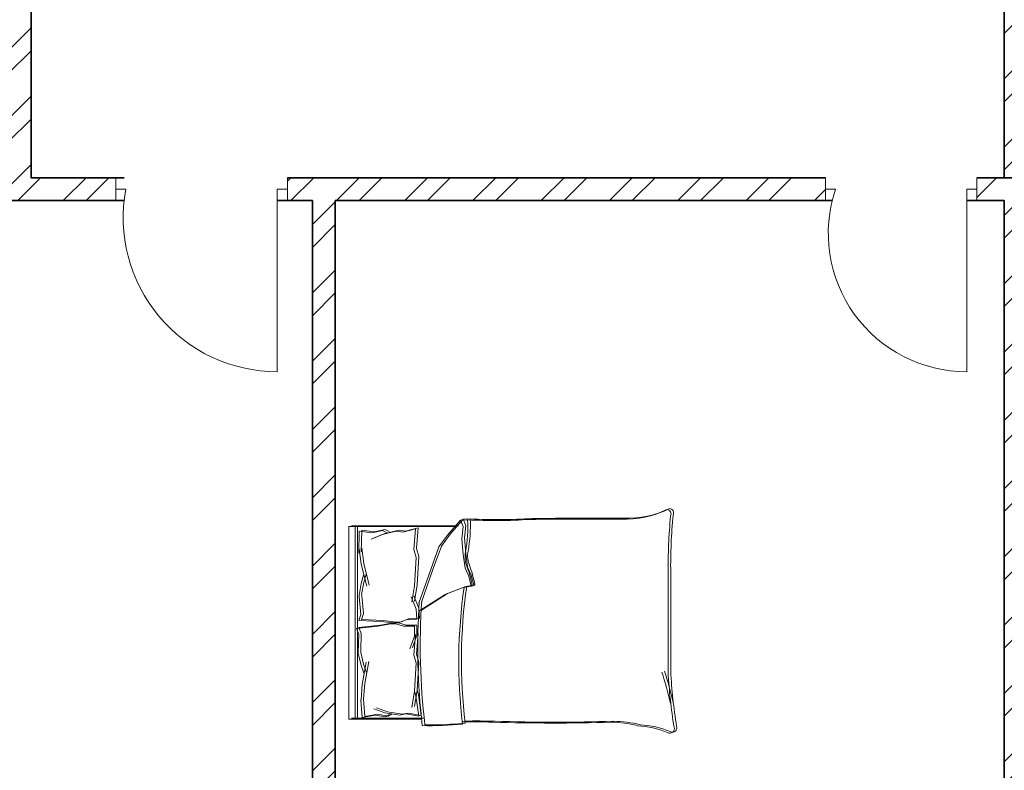
# Model space of a CAD drawing. Units: inches. Extents: x 1962 to 2771, y 1245 to 2660.
# Tile 3 of 114: x 2177 to 2371, y 1534 to 1683. Entities that reach past the tile are written whole.
import ezdxf

# ---------------------------------------------------------------- set-up
doc = ezdxf.new("R2010")
doc.units = ezdxf.units.IN
for name, color, linetype, lineweight in [('A-DOOR', 3, 'Continuous', 18), ('A-FURN', 8, 'Continuous', 13), ('A-WALL', 7, 'Continuous', 35), ('A-WALL-PATT', 252, 'Continuous', 13)]:
    doc.layers.add(name, color=color, linetype=linetype, lineweight=lineweight)

# ---------------------------------------------------------------- blocks, each defined once
blk = doc.blocks.new('BED-PLAN')
for p, q in [((0.51, 40.93), (21.66, 40.93)), ((0.51, 40.93), (21.66, 40.93)), ((1.73, 2.95), (1.73, 40.93)), ((1.73, 2.95), (1.73, 40.93)), ((22.05, 42.03), (19.47, 39.08)), ((22.05, 42.02), (19.47, 39.08)), ((22.56, 42.21), (19.98, 39.26)), ((22.56, 42.21), (19.98, 39.26)), ((23.44, 42.09), (22.05, 42.03, 3.08)), ((23.44, 42.09), (22.05, 42.02, 3.08)), ((22.55, 40.8), (22.05, 42.03)), ((22.55, 40.8), (22.05, 42.02)), ((22.3, 38.34), (22.55, 40.8)), ((22.3, 38.34), (22.55, 40.8)), ((23.95, 42.27), (22.56, 42.21, 3.08)), ((23.95, 42.27), (22.56, 42.21, 3.08)), ((23.06, 40.98), (22.56, 42.21)), ((23.06, 40.98), (22.56, 42.21)), ((22.81, 38.52), (23.06, 40.98)), ((22.81, 38.52), (23.06, 40.98)), ((0, 40.75), (21.15, 40.75)), ((0, 40.75), (21.15, 40.75)), ((0, 2.76), (0, 40.75)), ((1.22, 2.76), (1.22, 40.75)), ((1.22, 2.76), (1.22, 40.75)), ((2.03, 39.83), (1.96, 35.54)), ((2.03, 39.83), (1.96, 35.54)), ((2.03, 39.83), (4.58, 39.53)), ((2.03, 39.83), (4.58, 39.53)), ((2.54, 40.02), (2.46, 35.72)), ((2.54, 40.02), (2.46, 35.72)), ((2.54, 40.02), (5.09, 39.72)), ((2.54, 40.02), (5.09, 39.72)), ((6.56, 39.2), (4.43, 38.26)), ((6.56, 39.2), (4.43, 38.26)), ((4.58, 39.53), (6.63, 40.01)), ((4.58, 39.53), (6.63, 40.01)), ((7.07, 39.38), (4.94, 38.44)), ((7.07, 39.38), (4.94, 38.44)), ((5.09, 39.72), (7.14, 40.19)), ((5.09, 39.72), (7.14, 40.19)), ((9.4, 39.83), (6.56, 39.2)), ((9.4, 39.83), (6.56, 39.2)), ((6.63, 40.01), (7.46, 39.6)), ((6.63, 40.01), (7.46, 39.6)), ((9.91, 40.02), (7.07, 39.38)), ((9.91, 40.02), (7.07, 39.38)), ((7.14, 40.19), (7.97, 39.78)), ((7.14, 40.19), (7.97, 39.78)), ((10.68, 39.68), (9.4, 39.83)), ((10.68, 39.68), (9.4, 39.83)), ((11.19, 39.87), (9.91, 40.02)), ((11.19, 39.87), (9.91, 40.02)), ((13.17, 40.3), (10.68, 39.68)), ((13.17, 40.3), (10.68, 39.68)), ((13.68, 40.48), (11.19, 39.87)), ((13.68, 40.48), (11.19, 39.87)), ((12.85, 36.22), (13.17, 40.3)), ((12.85, 36.22), (13.17, 40.3)), ((13.36, 36.4), (13.68, 40.48)), ((13.36, 36.4), (13.68, 40.48)), ((19.47, 39.08), (17.75, 36.74)), ((19.47, 39.08), (17.75, 36.74)), ((19.98, 39.26), (18.26, 36.92)), ((19.98, 39.26), (18.26, 36.92)), ((18.26, 36.92), (16.66, 32.49)), ((18.26, 36.92), (16.66, 32.49)), ((22.55, 35.26), (22.3, 38.34)), ((22.55, 35.26), (22.3, 38.34)), ((23.06, 35.45), (22.81, 38.52)), ((23.06, 35.44), (22.81, 38.52)), ((1.96, 35.54), (2.02, 36.34)), ((1.96, 35.54), (2.02, 36.34)), ((2.02, 36.34), (2.44, 33.32)), ((2.02, 36.34), (2.44, 33.32)), ((2.46, 35.72), (2.53, 36.52)), ((2.46, 35.72), (2.53, 36.52)), ((2.53, 36.52), (2.95, 33.5)), ((2.53, 36.52), (2.95, 33.5)), ((13.3, 34.66), (12.85, 36.22)), ((13.3, 34.66), (12.85, 36.22)), ((13.8, 34.84), (13.36, 36.4)), ((13.8, 34.84), (13.36, 36.4)), ((17.75, 36.74), (16.15, 32.31)), ((17.75, 36.74), (16.15, 32.31)), ((22.92, 32.56), (22.55, 35.26)), ((22.92, 32.55), (22.55, 35.26)), ((23.42, 32.74), (23.06, 35.45)), ((23.42, 32.74), (23.06, 35.44)), ((2.44, 33.32), (3.52, 29.01)), ((2.44, 33.32), (3.52, 29.01)), ((2.95, 33.5), (4.02, 29.19)), ((2.95, 33.5), (4.02, 29.19)), ((12.95, 29.09), (13.3, 34.66)), ((12.95, 29.09), (13.3, 34.66)), ((13.46, 29.27), (13.8, 34.84)), ((13.46, 29.27), (13.8, 34.84)), ((2.92, 31.16), (2.45, 29.52)), ((2.92, 31.16), (2.45, 29.52)), ((3.43, 31.34), (2.96, 29.7)), ((3.43, 31.34), (2.96, 29.7)), ((16.15, 32.31), (13.82, 25.68)), ((16.15, 32.31), (13.82, 25.68)), ((16.66, 32.49), (14.33, 25.86)), ((16.66, 32.49), (14.33, 25.86)), ((23.65, 30.95), (22.92, 32.56)), ((23.65, 30.95), (22.92, 32.55)), ((24.16, 31.14), (23.42, 32.74)), ((24.16, 31.14), (23.42, 32.74)), ((24.65, 29.17), (24.16, 31.14)), ((24.65, 29.17), (24.16, 31.14)), ((62.99, 11.98), (62.99, 31.54)), ((62.99, 11.97), (62.99, 31.54)), ((63.5, 12.16), (63.5, 31.72)), ((63.5, 12.16), (63.5, 31.72)), ((2.45, 29.52), (2.02, 27.19)), ((2.45, 29.52), (2.02, 27.19)), ((2.96, 29.7), (2.52, 27.37)), ((2.96, 29.7), (2.52, 27.37)), ((12.93, 26.07), (13.46, 29.27)), ((12.93, 26.07), (13.46, 29.27)), ((23.06, 28.92), (24.65, 29.17)), ((23.06, 28.92), (24.65, 29.17)), ((24.15, 28.99), (23.65, 30.95)), ((24.15, 28.98), (23.65, 30.95)), ((2.52, 27.37), (2.54, 27.12)), ((2.52, 27.37), (2.54, 27.12)), ((12.42, 25.89), (12.95, 29.09)), ((12.42, 25.89), (12.95, 29.09)), ((13.82, 24.05), (18.98, 27.38)), ((13.82, 24.05), (18.98, 27.38)), ((14.33, 24.24), (19.49, 27.57)), ((14.33, 24.24), (19.49, 27.57)), ((18.98, 27.38), (22.55, 28.74)), ((18.98, 27.38), (22.55, 28.74)), ((19.49, 27.57), (23.06, 28.92)), ((19.49, 27.57), (23.06, 28.92)), ((22.55, 28.74), (24.15, 28.99)), ((22.55, 28.74), (24.15, 28.98)), ((2.02, 27.19), (2.03, 26.94)), ((2.02, 27.19), (2.03, 26.93)), ((2.03, 26.94), (2.37, 23.42)), ((2.03, 26.93), (2.37, 23.42)), ((2.54, 27.12), (2.88, 23.6)), ((2.54, 27.12), (2.88, 23.6)), ((13.31, 24.44), (12.28, 26.89)), ((13.31, 24.44), (12.28, 26.88)), ((13.81, 24.63), (12.79, 27.07)), ((13.81, 24.63), (12.79, 27.07)), ((2.37, 23.42), (1.98, 22.24)), ((2.37, 23.42), (1.98, 22.24)), ((2.88, 23.6), (2.49, 22.42)), ((2.88, 23.6), (2.49, 22.42)), ((13.43, 22.49), (13.31, 24.44)), ((13.43, 22.49), (13.31, 24.44)), ((13.94, 22.68), (13.81, 24.63)), ((13.94, 22.68), (13.81, 24.63)), ((1.98, 22.24), (6.25, 22.05)), ((1.98, 22.24), (6.25, 22.05)), ((2.49, 22.42), (6.76, 22.23)), ((2.49, 22.42), (6.76, 22.23)), ((5.74, 21.11), (8.27, 21.57)), ((5.74, 21.11), (8.27, 21.57)), ((6.25, 22.05), (8.81, 21.75)), ((6.25, 22.05), (8.81, 21.75)), ((6.25, 21.3), (8.78, 21.76)), ((6.25, 21.3), (8.78, 21.76)), ((6.76, 22.23), (9.31, 21.93)), ((6.76, 22.23), (9.31, 21.93)), ((8.27, 21.57), (9.3, 21.57)), ((8.27, 21.57), (9.3, 21.57)), ((8.78, 21.76), (9.81, 21.76)), ((8.78, 21.76), (9.81, 21.76)), ((8.81, 21.75), (9.84, 21.81)), ((8.81, 21.75), (9.84, 21.81)), ((9.3, 21.57), (10.8, 21.11)), ((9.3, 21.57), (10.8, 21.11)), ((9.31, 21.93), (10.35, 21.99)), ((9.31, 21.93), (10.35, 21.99)), ((9.81, 21.76), (11.3, 21.3)), ((9.81, 21.76), (11.3, 21.3)), ((9.84, 21.81), (11.3, 22.36)), ((9.84, 21.81), (11.3, 22.36)), ((10.35, 21.99), (11.81, 22.54)), ((10.35, 21.99), (11.81, 22.54)), ((11.3, 22.36), (13.43, 22.49)), ((11.3, 22.36), (13.43, 22.49)), ((11.81, 22.54), (13.94, 22.68)), ((11.81, 22.54), (13.94, 22.68)), ((1.49, 20.65), (5.74, 21.11)), ((1.49, 20.65), (5.74, 21.11)), ((1.95, 19.51), (1.49, 20.65)), ((1.95, 19.51), (1.49, 20.65)), ((1.83, 15.97), (1.95, 19.51)), ((1.83, 15.97), (1.95, 19.51)), ((1.99, 20.84), (6.25, 21.3)), ((1.99, 20.84), (6.25, 21.3)), ((2.45, 19.69), (1.99, 20.84)), ((2.45, 19.69), (1.99, 20.84)), ((2.34, 16.15), (2.45, 19.69)), ((2.34, 16.15), (2.45, 19.69)), ((10.8, 21.11), (12.93, 21.11)), ((10.8, 21.11), (12.93, 21.11)), ((11.3, 21.3), (13.44, 21.3)), ((11.3, 21.3), (13.44, 21.3)), ((12.85, 15.41), (13.17, 19.49)), ((12.85, 15.41), (13.17, 19.49)), ((12.93, 21.11), (12.93, 19.16)), ((12.93, 21.11), (12.93, 19.16)), ((13.36, 15.59), (13.68, 19.67)), ((13.36, 15.59), (13.68, 19.67)), ((13.44, 21.3), (13.44, 19.34)), ((13.44, 21.3), (13.44, 19.34)), ((12.93, 19.16), (12.06, 16.66)), ((12.93, 19.16), (12.06, 16.66)), ((13.44, 19.34), (12.57, 16.84)), ((13.44, 19.34), (12.57, 16.84)), ((1.83, 15.72), (1.83, 15.97)), ((1.83, 15.72), (1.83, 15.97)), ((2.41, 13.42), (1.83, 15.72)), ((2.41, 13.42), (1.83, 15.72)), ((2.34, 15.9), (2.34, 16.15)), ((2.34, 15.9), (2.34, 16.15)), ((2.91, 13.6), (2.34, 15.9)), ((2.91, 13.6), (2.34, 15.9)), ((13.8, 14.03), (13.36, 15.59)), ((13.8, 14.03), (13.36, 15.59)), ((2.64, 9.63), (3.44, 13.99)), ((2.64, 9.63), (3.44, 13.99)), ((3.49, 11.99), (2.91, 13.6)), ((3.49, 11.99), (2.91, 13.6)), ((3.14, 9.81), (3.95, 14.17)), ((3.14, 9.81), (3.95, 14.17)), ((13.3, 13.85), (12.85, 15.41)), ((13.3, 13.85), (12.85, 15.41)), ((12.95, 8.28), (13.3, 13.85)), ((12.95, 8.28), (13.3, 13.85)), ((13.46, 8.46), (13.8, 14.03)), ((13.46, 8.46), (13.8, 14.03)), ((2.98, 11.81), (2.41, 13.42)), ((2.98, 11.81), (2.41, 13.42)), ((2.91, 6.77), (3.14, 9.81)), ((2.91, 6.77), (3.14, 9.81)), ((2.41, 6.59), (2.64, 9.63)), ((2.41, 6.59), (2.64, 9.63)), ((12.42, 5.07), (12.95, 8.28)), ((12.42, 5.07), (12.95, 8.28)), ((12.93, 5.26), (13.46, 8.46)), ((12.93, 5.26), (13.46, 8.46)), ((12.95, 8.28), (13.21, 7.38)), ((12.95, 8.28), (13.21, 7.38)), ((13.46, 8.46), (13.72, 7.56)), ((13.46, 8.46), (13.72, 7.56)), ((2.39, 6.5), (2.41, 6.59)), ((2.39, 6.5), (2.41, 6.59)), ((2.65, 3.1), (2.39, 6.5)), ((2.65, 3.1), (2.39, 6.5)), ((2.9, 6.68), (2.91, 6.77)), ((2.9, 6.68), (2.91, 6.77)), ((3.16, 3.28), (2.9, 6.68)), ((3.16, 3.28), (2.9, 6.68)), ((13.21, 7.38), (13.78, 3.33)), ((13.21, 7.38), (13.78, 3.33)), ((13.72, 7.56), (14.29, 3.51)), ((13.72, 7.56), (14.29, 3.51)), ((7.12, 4.02), (4.93, 4.82)), ((7.12, 4.02), (4.93, 4.82)), ((7.63, 4.2), (5.44, 5)), ((7.63, 4.2), (5.44, 5)), ((9.99, 3.56), (7.12, 4.02)), ((9.99, 3.56), (7.12, 4.02)), ((10.5, 3.74), (7.63, 4.2)), ((10.5, 3.74), (7.63, 4.2)), ((11.76, 3.97), (10.5, 3.74)), ((11.76, 3.97), (10.5, 3.74)), ((14.29, 3.51), (11.76, 3.97)), ((14.29, 3.51), (11.76, 3.97)), ((14.4, 2.76), (0, 2.76)), ((14.4, 2.76), (0, 2.76)), ((14.9, 2.95), (0.51, 2.95)), ((14.9, 2.95), (0.51, 2.95)), ((2.64, 3.1), (5.16, 3.56)), ((2.64, 3.1), (5.16, 3.56)), ((3.14, 3.28), (5.67, 3.74)), ((3.14, 3.28), (5.67, 3.74)), ((5.16, 3.56), (7.23, 3.21)), ((5.16, 3.56), (7.23, 3.21)), ((5.67, 3.74), (7.74, 3.39)), ((5.67, 3.74), (7.74, 3.39)), ((7.23, 3.21), (8.04, 3.67)), ((7.23, 3.21), (8.04, 3.67)), ((7.74, 3.39), (8.55, 3.85)), ((7.74, 3.39), (8.55, 3.85)), ((11.26, 3.79), (9.99, 3.56)), ((11.26, 3.79), (9.99, 3.56)), ((13.78, 3.33), (11.26, 3.79)), ((13.78, 3.33), (11.26, 3.79))]:
    blk.add_line(p, q)
for centre, radius, start, end in [((54.58, 60.54), 18.33, 267.4714, 296.4681), ((54.58, 60.54), 18.33, 267.4714, 296.4681), ((55.09, 60.72), 18.33, 267.4714, 296.4681), ((55.09, 60.72), 18.33, 267.4714, 296.4681), ((62.69, 43.25), 0.876, 332.6588, 86.02), ((62.69, 43.25), 0.876, 332.6588, 86.02), ((168.74, 32.71), 105.75, 174.4998, 180.6351), ((168.74, 32.71), 105.75, 174.4998, 180.6351), ((63.2, 43.43), 0.876, 332.6588, 86.02), ((63.2, 43.43), 0.876, 332.6588, 86.02), ((169.24, 32.89), 105.75, 174.4998, 180.6351), ((169.24, 32.89), 105.75, 174.4998, 180.6351), ((-5.29, 40.8), 28.76, 349.8763, 2.5657), ((-5.29, 40.8), 28.76, 349.8763, 2.5657), ((28.87, 144.88), 102.94, 266.9791, 273.8365), ((28.87, 144.88), 102.94, 266.9791, 273.8365), ((-4.78, 40.98), 28.76, 349.8763, 2.5657), ((-4.78, 40.98), 28.76, 349.8763, 2.5657), ((29.37, 145.06), 102.94, 266.9791, 273.8365), ((29.37, 145.06), 102.94, 266.9791, 273.8365), ((53.91, -3583.94), 3626.16, 90.00217, 90.28689), ((53.91, -3583.94), 3626.16, 90.00217, 90.28689), ((54.42, -3583.75), 3626.16, 90.00217, 90.28689), ((54.42, -3583.75), 3626.16, 90.00217, 90.28689), ((27.87, 34.77), 4.95, 168.6608, 203.7384), ((27.87, 34.77), 4.95, 168.6608, 203.7384), ((28.38, 34.95), 4.95, 168.6608, 203.7384), ((28.38, 34.95), 4.95, 168.6608, 203.7384), ((1.18, 24.77), 23.57, 10.6617, 19.8806), ((1.18, 24.76), 23.57, 10.6617, 19.8806), ((1.69, 24.95), 23.57, 10.6617, 19.8806), ((1.69, 24.95), 23.57, 10.6617, 19.8806), ((24.7, 29.3), 0.147, 250.2464, 1.1377), ((24.7, 29.3), 0.147, 250.2464, 1.1377), ((124.25, 14.12), 102.56, 171.7845, 186.9006), ((124.25, 14.11), 102.56, 171.7845, 186.9006), ((124.76, 14.3), 102.56, 171.7845, 186.9006), ((124.76, 14.3), 102.56, 171.7845, 186.9006), ((24.2, 29.12), 0.147, 250.2464, 1.1377), ((24.2, 29.12), 0.147, 250.2464, 1.1377), ((144.71, 16.98), 131.13, 176.0865, 186.7821), ((144.71, 16.98), 131.13, 176.0865, 186.7821), ((145.22, 17.16), 131.13, 176.0865, 186.7821), ((145.22, 17.16), 131.13, 176.0865, 186.7821), ((-18.85, -13.69), 84.62, 13.3832, 17.7053), ((-18.85, -13.69), 84.62, 13.3832, 17.7053), ((-18.34, -13.51), 84.62, 13.3832, 17.7053), ((-18.34, -13.51), 84.62, 13.3832, 17.7053), ((159.64, 17.03), 96.78, 182.9958, 189.4091), ((159.64, 17.03), 96.78, 182.9958, 189.4091), ((160.15, 17.21), 96.78, 182.9958, 189.4091), ((160.15, 17.21), 96.78, 182.9958, 189.4091), ((16.48, 67.88), 66.22, 268.7218, 275.604), ((16.48, 67.88), 66.22, 268.7218, 275.604), ((24.78, -132.99), 135.22, 88.4762, 91.0082), ((24.78, -132.99), 135.22, 88.4762, 91.0082), ((25.29, -132.81), 135.22, 88.4762, 91.0082), ((25.29, -132.81), 135.22, 88.4762, 91.0082), ((40.23, 385.38), 383.38, 268.2277, 271.7185), ((40.23, 385.38), 383.38, 268.2277, 271.7185), ((40.74, 385.56), 383.38, 268.2277, 271.7185), ((40.74, 385.56), 383.38, 268.2277, 271.7185), ((51.28, -21.38), 23.56, 76.0648, 88.9113), ((51.28, -21.38), 23.56, 76.0648, 88.9113), ((51.79, -21.2), 23.56, 76.0648, 88.9113), ((51.79, -21.2), 23.56, 76.0648, 88.9113), ((15.97, 67.7), 66.22, 268.7218, 275.604), ((15.97, 67.7), 66.22, 268.7218, 275.604), ((55.86, -17.22), 18.73, 67.9751, 86.652), ((55.86, -17.22), 18.73, 67.9751, 86.652), ((56.37, -17.03), 18.73, 67.9751, 86.652), ((56.37, -17.03), 18.73, 67.9751, 86.652), ((63.37, 0.87), 0.866, 236.1736, 23.4781), ((63.37, 0.87), 0.866, 236.1736, 23.4781), ((63.87, 1.05), 0.866, 236.1736, 23.4781), ((63.87, 1.05), 0.866, 236.1736, 23.4781)]:
    blk.add_arc(centre, radius, start, end)

msp = doc.modelspace()

# ---------------------------------------------------------------- hatches: boundary and pattern name
at = {"layer": 'A-WALL-PATT'}
h = msp.add_hatch(dxfattribs=at)
h.set_pattern_fill('ANSI32', color=256)
h.paths.add_polyline_path([(2090.8074, 2467.3437), (2141.6481, 2467.3437), (2141.6481, 2469.5937), (2141.6481, 2471.8437), (2086.3074, 2471.8437), (2086.3074, 2422.5333), (2090.8074, 2422.5333)])
h.paths.add_polyline_path([(2282.7664, 2471.8437), (2204.8982, 2471.8437), (2204.8982, 2467.3437), (2234.8074, 2467.3437), (2234.8074, 2311.3437), (2228.7492, 2311.3437), (2228.7492, 2306.8437), (2234.8074, 2306.8437), (2331.9227, 2306.8437), (2331.9227, 2309.0937), (2331.9227, 2311.3437), (2239.3074, 2311.3437), (2239.3074, 2467.3437), (2282.7664, 2467.3437), (2282.7664, 2469.5937)])
h.paths.add_polyline_path([(2471.4531, 2519.8437), (2552.011, 2519.8437), (2564.3996, 2519.8437), (2564.3996, 2511.1389), (2568.8996, 2511.1389), (2568.8996, 2524.3437), (2466.9531, 2524.3437), (2466.9531, 2471.8437), (2450.0749, 2471.8437), (2446.4672, 2471.8437), (2446.4672, 2467.3437), (2450.0749, 2467.3437), (2475.9988, 2467.3437), (2475.9988, 2469.5937), (2475.9988, 2471.8437), (2471.4531, 2471.8437)])
h.paths.add_polyline_path([(2575.2231, 2469.5937), (2575.2231, 2471.8437), (2568.8996, 2471.8437), (2568.8996, 2487.1389), (2564.3996, 2487.1389), (2564.3996, 2471.8437), (2556.511, 2471.8437), (2499.2904, 2471.8437), (2499.2904, 2467.3437), (2507.8074, 2467.3437), (2507.8074, 2311.3437), (2414.863, 2311.3437), (2414.863, 2306.8437), (2512.3074, 2306.8437), (2517.0114, 2306.8437), (2517.0114, 2309.0937), (2517.0114, 2311.3437), (2512.3074, 2311.3437), (2512.3074, 2467.3437), (2575.2231, 2467.3437)])
h.paths.add_polyline_path([(2660.8074, 2471.8437), (2600.9602, 2471.8437), (2600.9602, 2467.3437), (2656.3074, 2467.3437), (2656.3074, 2432.5704), (2660.8074, 2432.5704)])
h.paths.add_polyline_path([(2660.8074, 2372.5704), (2656.3074, 2372.5704), (2656.3074, 2311.3437), (2600.276, 2311.3437), (2600.276, 2309.0937), (2600.276, 2306.8437), (2656.3074, 2306.8437), (2656.3074, 2296.2593), (2660.8074, 2296.2593)])
h.paths.add_polyline_path([(2572.3074, 2306.8437), (2577.1385, 2306.8437), (2577.1385, 2311.3437), (2551.082, 2311.3437), (2551.082, 2306.8437), (2567.8074, 2306.8437), (2567.8074, 2258.8437), (2540.0574, 2258.8437), (2540.0574, 2256.5937), (2540.0574, 2254.3437), (2567.8074, 2254.3437), (2656.3074, 2254.3437), (2656.3074, 2236.9085), (2660.8074, 2236.9085), (2660.8074, 2272.2593), (2656.3074, 2272.2593), (2656.3074, 2258.8437), (2572.3074, 2258.8437)])
h.paths.add_polyline_path([(2512.3074, 2254.3437), (2518.8716, 2254.3437), (2518.8716, 2256.5937), (2518.8716, 2258.8437), (2507.8074, 2258.8437), (2507.8074, 2177.8437), (2567.8074, 2177.8437), (2567.8074, 2172.9628), (2572.3074, 2172.9628), (2572.3074, 2177.8437), (2656.3074, 2177.8437), (2656.3074, 2166.4846), (2660.8074, 2166.4846), (2660.8074, 2200.9085), (2656.3074, 2200.9085), (2656.3074, 2182.3437), (2512.3074, 2182.3437)])
h.paths.add_polyline_path([(2656.3074, 2129.8437), (2572.3074, 2129.8437), (2572.3074, 2150.3044), (2570.0574, 2150.3044), (2567.8074, 2150.3044), (2567.8074, 2129.8437), (2507.8074, 2129.8437), (2507.8074, 2116.3027), (2510.0574, 2116.3027), (2512.3074, 2116.3027), (2512.3074, 2125.3437), (2567.8074, 2125.3437), (2572.3074, 2125.3437), (2656.3074, 2125.3437)])
h.paths.add_polyline_path([(2090.8074, 2362.5333), (2086.3074, 2362.5333), (2086.3074, 2298.6242), (2090.8074, 2298.6242), (2090.8074, 2306.8437), (2174.8074, 2306.8437), (2174.8074, 2286.4178), (2179.3074, 2286.4178), (2179.3074, 2306.8437), (2192.8641, 2306.8437), (2192.8641, 2309.0937), (2192.8641, 2311.3437), (2090.8074, 2311.3437)])
h.paths.add_polyline_path([(2209.156, 2258.8437), (2179.3074, 2258.8437), (2179.3074, 2263.2236), (2177.0574, 2263.2236), (2174.8074, 2263.2236), (2174.8074, 2258.8437), (2090.8074, 2258.8437), (2090.8074, 2274.6242), (2086.3074, 2274.6242), (2086.3074, 2238.2967), (2088.5574, 2238.2967), (2090.8074, 2238.2967), (2090.8074, 2254.3437), (2209.156, 2254.3437)])
h.paths.add_polyline_path([(2090.8074, 2177.8437), (2234.8074, 2177.8437), (2234.8074, 2173.1428), (2239.3074, 2173.1428), (2239.3074, 2258.8437), (2230.8442, 2258.8437), (2230.8442, 2256.5937), (2230.8442, 2254.3437), (2234.8074, 2254.3437), (2234.8074, 2182.3437), (2090.8074, 2182.3437), (2090.8074, 2202.2967), (2086.3074, 2202.2967), (2086.3074, 2140.0389), (2090.8074, 2140.0389)])
h.paths.add_polyline_path([(2090.8074, 2080.0389), (2086.3074, 2080.0389), (2086.3074, 2033.8437), (2090.8074, 2033.8437)], flags=17)
h.paths.add_polyline_path([(2244.9405, 2033.8437), (2239.3074, 2033.8437), (2239.3074, 2142.0665), (2237.2592, 2142.0665), (2234.8074, 2142.0665), (2234.8074, 2033.8437), (2090.8074, 2033.8437), (2076.5204, 2033.8437), (2072.0204, 2033.8437), (2072.0204, 2000.4493), (2076.5204, 2000.4493), (2076.5204, 2029.3437), (2090.8074, 2029.3437), (2244.9405, 2029.3437), (2244.9405, 2031.5937)])
h.paths.add_polyline_path([(2234.8074, 1933.3437), (2076.5204, 1933.3437), (2076.5204, 1952.4493), (2074.2704, 1952.4493), (2072.0204, 1952.4493), (2072.0204, 1933.3437), (2072.0204, 1928.8437), (2234.8074, 1928.8437)])
h.paths.add_polyline_path([(2090.8074, 1928.8437), (2086.3074, 1928.8437), (2086.3074, 1906.5013), (2090.8074, 1906.5013)])
h.paths.add_polyline_path([(2090.8074, 1846.5013), (2086.3074, 1846.5013), (2086.3074, 1769.9917), (2088.5574, 1769.9917), (2090.8074, 1769.9917), (2090.8074, 1780.3437), (2234.8074, 1780.3437), (2234.8074, 1708.3437), (2230.3764, 1708.3437), (2230.3764, 1703.8437), (2239.3074, 1703.8437), (2239.3074, 1792.6669), (2237.0574, 1792.6669), (2234.8074, 1792.6669), (2234.8074, 1784.8437), (2090.8074, 1784.8437)])
h.paths.add_polyline_path([(2239.3074, 1928.8437), (2244.9405, 1928.8437), (2244.9405, 1931.0937), (2244.9405, 1933.3437), (2234.8074, 1933.3437), (2234.8074, 1928.8437), (2234.8074, 1825.5949), (2239.3074, 1825.5949)])
h.paths.add_polyline_path([(2148.0425, 1649.0937), (2148.0425, 1651.3437), (2090.8074, 1651.3437), (2090.8074, 1646.8437), (2148.0425, 1646.8437)], flags=0)
h.paths.add_polyline_path([(2207.5601, 1708.3437), (2090.8074, 1708.3437), (2090.8074, 1703.8437), (2174.8074, 1703.8437), (2174.8074, 1651.3437), (2170.4457, 1651.3437), (2170.4457, 1646.8437), (2195.9924, 1646.8437), (2195.9924, 1649.0937), (2195.9924, 1651.3437), (2179.3074, 1651.3437), (2179.3074, 1703.8437), (2207.5601, 1703.8437), (2207.5601, 1706.0937)])
h.paths.add_polyline_path([(2090.8074, 1733.9917), (2086.3074, 1733.9917), (2086.3074, 1696.1032), (2088.5574, 1696.1032), (2090.8074, 1696.1032)])
h.paths.add_polyline_path([(2090.8074, 1672.1032), (2086.3074, 1672.1032), (2086.3074, 1600.3335), (2090.8074, 1600.3335)])
h.paths.add_polyline_path([(2090.8074, 1540.3335), (2086.3074, 1540.3335), (2086.3074, 1486.3437), (2139.6766, 1486.3437), (2139.6766, 1490.8437), (2090.8074, 1490.8437)])
h.paths.add_polyline_path([(2302.3876, 1490.8437), (2239.3074, 1490.8437), (2239.3074, 1646.8437), (2335.9994, 1646.8437), (2335.9994, 1651.3437), (2229.884, 1651.3437), (2229.884, 1646.8437), (2234.8074, 1646.8437), (2234.8074, 1490.8437), (2202.7103, 1490.8437), (2202.7103, 1488.5937), (2202.7103, 1486.3437), (2275.0699, 1486.3437), (2275.0699, 1475.772), (2279.5699, 1475.772), (2279.5699, 1486.3437), (2302.3876, 1486.3437)])
h.paths.add_polyline_path([(2279.5699, 1451.772), (2275.0699, 1451.772), (2275.0699, 1438.3437), (2174.8074, 1438.3437), (2174.8074, 1486.3437), (2179.7922, 1486.3437), (2179.7922, 1490.8437), (2163.3585, 1490.8437), (2163.3585, 1488.5937), (2163.3585, 1486.3437), (2170.3074, 1486.3437), (2170.3074, 1433.8437), (2279.5699, 1433.8437)])
h.paths.add_polyline_path([(2427.2363, 1490.8437), (2375.8074, 1490.8437), (2375.8074, 1646.8437), (2381.6401, 1646.8437), (2381.6401, 1651.3437), (2365.887, 1651.3437), (2365.887, 1649.0937), (2365.887, 1646.8437), (2371.3074, 1646.8437), (2371.3074, 1490.8437), (2327.5627, 1490.8437), (2327.5627, 1488.5937), (2327.5627, 1486.3437), (2371.3074, 1486.3437), (2371.3074, 1433.8437), (2375.8074, 1433.8437), (2375.8074, 1486.3437), (2427.2363, 1486.3437)])
h.paths.add_polyline_path([(2512.3074, 1646.8437), (2519.4351, 1646.8437), (2519.4351, 1649.0937), (2519.4351, 1651.3437), (2507.8074, 1651.3437), (2416.0063, 1651.3437), (2416.0063, 1649.0937), (2416.0063, 1646.8437), (2507.8074, 1646.8437), (2507.8074, 1490.8437), (2497.0532, 1490.8437), (2497.0532, 1488.5937), (2497.0532, 1486.3437), (2574.9344, 1486.3437), (2574.9344, 1476.0181), (2579.4344, 1476.0181), (2579.4344, 1486.3437), (2584.4872, 1486.3437), (2584.3074, 1490.8437), (2512.3074, 1490.8437)])
h.paths.add_polyline_path([(2470.5091, 1486.3437), (2473.9767, 1486.3437), (2473.9767, 1490.8437), (2449.6605, 1490.8437), (2449.6605, 1488.5937), (2449.6605, 1486.3437), (2466.0091, 1486.3437), (2466.0091, 1433.8437), (2470.5091, 1433.8437), (2579.4344, 1433.8437), (2579.4344, 1452.0181), (2574.9344, 1452.0181), (2574.9344, 1438.3437), (2554.5091, 1438.3437), (2470.5091, 1438.3437)])
h.paths.add_polyline_path([(2656.3074, 1490.8437), (2611.86, 1490.8437), (2611.86, 1486.3437), (2656.3074, 1486.3437)])
h.paths.add_polyline_path([(2660.8074, 1532.7007), (2658.5574, 1532.7007), (2656.3074, 1532.7007), (2656.3074, 1486.3437), (2660.8074, 1486.3437)])
h.paths.add_polyline_path([(2660.8074, 1664.9663), (2656.3074, 1664.9663), (2656.3074, 1651.3437), (2602.2313, 1651.3437), (2602.2313, 1646.8437), (2656.3074, 1646.8437), (2656.3074, 1592.7007), (2660.8074, 1592.7007)])
h.paths.add_polyline_path([(2660.8074, 1724.5221), (2656.3074, 1724.5221), (2656.3074, 1703.8437), (2542.4725, 1703.8437), (2542.4725, 1699.3437), (2567.8074, 1699.3437), (2567.8074, 1651.3437), (2552.7766, 1651.3437), (2552.7766, 1649.0937), (2552.7766, 1646.8437), (2577.2878, 1646.8437), (2577.2878, 1649.0937), (2577.2878, 1651.3437), (2572.3074, 1651.3437), (2572.3074, 1699.3437), (2656.3074, 1699.3437), (2656.3074, 1688.9663), (2660.8074, 1688.9663)])
h.paths.add_polyline_path([(2660.8074, 1880.6524), (2656.3074, 1880.6524), (2656.3074, 1832.8437), (2512.3074, 1832.8437), (2512.3074, 1837.8959), (2507.8074, 1837.8959), (2507.8074, 1828.3437), (2567.8074, 1828.3437), (2567.8074, 1804.3437), (2572.3074, 1804.3437), (2572.3074, 1828.3437), (2656.3074, 1828.3437), (2656.3074, 1818.6778), (2660.8074, 1818.6778)])
h.paths.add_polyline_path([(2660.8074, 1794.6778), (2656.3074, 1794.6778), (2656.3074, 1780.3437), (2572.3074, 1780.3437), (2572.3074, 1783.0303), (2570.0574, 1783.0303), (2567.8074, 1783.0303), (2567.8074, 1780.3437), (2507.8074, 1780.3437), (2507.8074, 1699.3437), (2517.8858, 1699.3437), (2517.8858, 1701.5937), (2517.8858, 1703.8437), (2512.3074, 1703.8437), (2512.3074, 1775.8437), (2656.3074, 1775.8437), (2656.3074, 1760.5221), (2660.8074, 1760.5221)])
h.paths.add_polyline_path([(2660.8074, 1981.3437), (2660.8074, 2020.2808), (2658.5574, 2020.2808), (2656.3074, 2020.2808), (2656.3074, 1981.3437), (2512.3074, 1981.3437), (2512.3074, 2086.6996), (2507.8074, 2086.6996), (2507.8074, 1981.3437), (2375.8074, 1981.3437), (2375.8074, 1986.8505), (2373.5574, 1986.8505), (2371.3074, 1986.8505), (2371.3074, 1973.2607), (2375.8074, 1973.2607), (2375.8074, 1976.8437), (2507.8074, 1976.8437), (2507.8074, 1865.4281), (2510.0574, 1865.4281), (2512.3074, 1865.4281), (2512.3074, 1976.8437), (2660.8074, 1976.8437)])
h.paths.add_polyline_path([(2375.8074, 1940.297), (2373.5574, 1940.297), (2371.3074, 1940.297), (2371.3074, 1933.3437), (2278.4434, 1933.3437), (2278.4434, 1928.8437), (2371.3074, 1928.8437), (2371.3074, 1651.3437), (2375.8074, 1651.3437)])
h.paths.add_polyline_path([(2660.8074, 1976.8437), (2656.3074, 1976.8437), (2656.3074, 1940.6524), (2660.8074, 1940.6524)], flags=17)
h.paths.add_polyline_path([(2660.8074, 2142.4846), (2656.3074, 2142.4846), (2656.3074, 2080.2808), (2660.8074, 2080.2808)])
h.paths.add_polyline_path([(2381.4189, 2311.3437), (2375.8074, 2311.3437), (2375.8074, 2467.3437), (2424.7242, 2467.3437), (2424.7242, 2469.5937), (2424.7242, 2471.8437), (2375.8074, 2471.8437), (2375.8074, 2524.3437), (2371.3074, 2524.3437), (2371.3074, 2471.8437), (2307.2097, 2471.8437), (2307.2097, 2467.3437), (2371.3074, 2467.3437), (2371.3074, 2311.3437), (2366.8901, 2311.3437), (2366.8901, 2306.8437), (2371.3074, 2306.8437), (2371.3074, 2033.8437), (2279.6589, 2033.8437), (2279.6589, 2029.3437), (2371.3074, 2029.3437), (2371.3074, 2014.2598), (2375.8074, 2014.2598), (2375.8074, 2306.8437), (2381.4189, 2306.8437)])
h.paths.add_polyline_path([(2263.3074, 2524.3437), (2170.3074, 2524.3437), (2170.3074, 2519.8437), (2170.3074, 2471.8437), (2165.0312, 2471.8437), (2165.0312, 2467.3437), (2179.6721, 2467.3437), (2179.6721, 2469.5161), (2179.6721, 2471.8437), (2174.8074, 2471.8437), (2174.8074, 2519.8437), (2258.8074, 2519.8437), (2258.8074, 2511.6436), (2263.3074, 2511.6436)])
h.paths.add_polyline_path([(2245.0232, 1361.4123), (2492.9468, 1361.4123), (2492.9468, 1398.505), (2245.0232, 1398.505)], flags=9)
h.paths.add_polyline_path([(2388.1434, 2086.6936), (2425.0704, 2086.6936), (2425.0704, 2105.3509), (2388.1434, 2105.3509)], flags=9)
h.paths.add_polyline_path([(2404.922, 2242.6744), (2445.7337, 2242.6744), (2445.7337, 2261.3318), (2404.922, 2261.3318)], flags=9)
h.paths.add_polyline_path([(2269.4107, 2156.7935), (2306.3378, 2156.7935), (2306.3378, 2175.4508), (2269.4107, 2175.4508)], flags=9)
h.paths.add_polyline_path([(2269.3277, 2233.4343), (2306.2547, 2233.4343), (2306.2547, 2252.0917), (2269.3277, 2252.0917)], flags=9)
h.paths.add_polyline_path([(2431.6052, 2320.6922), (2470.4456, 2320.6922), (2470.4456, 2339.3495), (2431.6052, 2339.3495)], flags=25)
h.paths.add_polyline_path([(2249.6902, 2315.7608), (2288.5306, 2315.7608), (2288.5306, 2334.4182), (2249.6902, 2334.4182)], flags=25)
h.paths.add_polyline_path([(2096.9301, 2314.3181), (2135.7704, 2314.3181), (2135.7704, 2332.9755), (2096.9301, 2332.9755)], flags=25)
h.paths.add_polyline_path([(2134.3475, 2285.7089), (2161.4655, 2285.7089), (2161.4655, 2304.3662), (2134.3475, 2304.3662)], flags=9)
h.paths.add_polyline_path([(2126.5155, 2209.4076), (2159.9227, 2209.4076), (2159.9227, 2228.065), (2126.5155, 2228.065)], flags=25)
h.paths.add_polyline_path([(2110.5753, 2141.5299), (2149.4157, 2141.5299), (2149.4157, 2160.1872), (2110.5753, 2160.1872)], flags=25)
h.paths.add_polyline_path([(2249.8618, 1968.3317), (2286.3966, 1968.3317), (2286.3966, 1986.989), (2249.8618, 1986.989)], flags=9)
h.paths.add_polyline_path([(2395.9507, 1777.0051), (2436.7624, 1777.0051), (2436.7624, 1795.6625), (2395.9507, 1795.6625)], flags=9)
h.paths.add_polyline_path([(2398.5259, 1888.5651), (2435.0062, 1888.5651), (2435.0062, 1907.2224), (2398.5259, 1907.2224)], flags=25)
h.paths.add_polyline_path([(2259.3506, 1728.3559), (2296.2776, 1728.3559), (2296.2776, 1747.0132), (2259.3506, 1747.0132)], flags=9)
h.paths.add_polyline_path([(2271.3698, 1845.268), (2308.2968, 1845.268), (2308.2968, 1863.9253), (2271.3698, 1863.9253)], flags=9)
h.paths.add_polyline_path([(2120.9355, 1786.3027), (2159.7759, 1786.3027), (2159.7759, 1804.9601), (2120.9355, 1804.9601)], flags=25)
h.paths.add_polyline_path([(2121.3164, 1732.1043), (2154.7236, 1732.1043), (2154.7236, 1750.7616), (2121.3164, 1750.7616)], flags=25)
h.paths.add_polyline_path([(2118.3706, 1678.8997), (2147.5282, 1678.8997), (2147.5282, 1697.557), (2118.3706, 1697.557)], flags=25)
h.paths.add_polyline_path([(2385.9227, 1493.557), (2424.763, 1493.557), (2424.763, 1512.2143), (2385.9227, 1512.2143)], flags=25)
h.paths.add_polyline_path([(2248.7058, 1500.0256), (2287.5462, 1500.0256), (2287.5462, 1518.6829), (2248.7058, 1518.6829)], flags=25)
h.paths.add_polyline_path([(2104.1669, 1617.3771), (2143.0073, 1617.3771), (2143.0073, 1636.0344), (2104.1669, 1636.0344)], flags=9)
h.paths.add_polyline_path([(2096.0714, 1447.8824), (2137.3845, 1447.8824), (2137.3845, 1458.1859), (2096.0714, 1458.1859)], flags=9)
h.paths.add_polyline_path([(2180.6114, 1440.325), (2209.7689, 1440.325), (2209.7689, 1458.9823), (2180.6114, 1458.9823)], flags=25)
h.paths.add_polyline_path([(2316.1698, 1447.9637), (2357.4829, 1447.9637), (2357.4829, 1458.2673), (2316.1698, 1458.2673)], flags=9)
h.paths.add_polyline_path([(2397.6187, 1447.9637), (2438.9318, 1447.9637), (2438.9318, 1458.2673), (2397.6187, 1458.2673)], flags=9)
h.paths.add_polyline_path([(2473.0778, 1439.5953), (2502.2354, 1439.5953), (2502.2354, 1458.2527), (2473.0778, 1458.2527)], flags=25)
h.paths.add_polyline_path([(2589.7027, 1447.8819), (2631.0158, 1447.8819), (2631.0158, 1458.1855), (2589.7027, 1458.1855)], flags=9)
h.paths.add_polyline_path([(2522.4009, 1497.5285), (2561.2413, 1497.5285), (2561.2413, 1516.1859), (2522.4009, 1516.1859)], flags=25)
h.paths.add_polyline_path([(2579.6565, 1671.3482), (2608.8141, 1671.3482), (2608.8141, 1690.0056), (2579.6565, 1690.0056)], flags=25)
h.paths.add_polyline_path([(2544.7038, 1725.5064), (2578.1111, 1725.5064), (2578.1111, 1744.1637), (2544.7038, 1744.1637)], flags=25)
h.paths.add_polyline_path([(2578.1191, 1807.472), (2607.2766, 1807.472), (2607.2766, 1826.1293), (2578.1191, 1826.1293)], flags=25)
h.paths.add_polyline_path([(2595.0614, 1835.1839), (2633.9018, 1835.1839), (2633.9018, 1853.8413), (2595.0614, 1853.8413)], flags=25)
h.paths.add_polyline_path([(2567.0097, 2097.7035), (2605.8501, 2097.7035), (2605.8501, 2116.3609), (2567.0097, 2116.3609)], flags=9)
h.paths.add_polyline_path([(2586.644, 2134.6454), (2615.8015, 2134.6454), (2615.8015, 2153.3027), (2586.644, 2153.3027)], flags=9)
h.paths.add_polyline_path([(2544.6185, 2212.6783), (2578.0258, 2212.6783), (2578.0258, 2231.3356), (2544.6185, 2231.3356)], flags=25)
h.paths.add_polyline_path([(2577.0273, 2256.9023), (2606.1849, 2256.9023), (2606.1849, 2275.5597), (2577.0273, 2275.5597)], flags=24)
h.paths.add_polyline_path([(2605.2683, 2315.2821), (2644.1087, 2315.2821), (2644.1087, 2333.9395), (2605.2683, 2333.9395)], flags=25)
h.paths.add_polyline_path([(2583.1244, 2496.1815), (2624.4375, 2496.1815), (2624.4375, 2506.4851), (2583.1244, 2506.4851)], flags=9)
h.paths.add_polyline_path([(2474.761, 2497.0823), (2503.9185, 2497.0823), (2503.9185, 2515.7397), (2474.761, 2515.7397)], flags=25)
h.paths.add_polyline_path([(2387.5787, 2494.2563), (2428.902, 2494.2563), (2428.902, 2504.5598), (2387.5787, 2504.5598)], flags=9)
h.paths.add_polyline_path([(2300.1657, 2500.1564), (2341.4788, 2500.1564), (2341.4788, 2510.46), (2300.1657, 2510.46)], flags=25)
h.paths.add_polyline_path([(2176.8589, 2497.5843), (2206.0165, 2497.5843), (2206.0165, 2516.2416), (2176.8589, 2516.2416)], flags=25)
h.paths.add_polyline_path([(2097.4668, 2494.9762), (2138.7799, 2494.9762), (2138.7799, 2505.2798), (2097.4668, 2505.2798)], flags=9)

# ---------------------------------------------------------------- linework, layer by layer
at = {"layer": 'A-DOOR'}
for p, q in [((2195.9924, 1651.3437), (2195.9924, 1646.8437)), ((2229.884, 1649.1113), (2229.884, 1651.3437)), ((2229.884, 1651.3437), (2229.884, 1646.8437)), ((2335.9994, 1646.8437), (2335.9994, 1651.3437)), ((2335.9994, 1651.3437), (2335.9994, 1649.0937)), ((2365.887, 1646.8437), (2365.887, 1651.3437)), ((2365.887, 1651.3437), (2365.887, 1649.0937)), ((2195.9924, 1646.8437), (2195.9924, 1649.0937)), ((2195.9924, 1649.0937), (2197.9924, 1649.0937)), ((2227.884, 1613.0937), (2227.884, 1649.1113)), ((2227.884, 1649.1113), (2229.884, 1649.1113)), ((2335.9994, 1649.0937), (2337.9994, 1649.0937)), ((2365.887, 1649.0937), (2363.887, 1649.0937)), ((2363.887, 1649.0937), (2363.887, 1613.0937))]:
    msp.add_line(p, q, dxfattribs=at)
for centre, radius, start in [((2227.884, 1643.5035), 30.4098, 169.407211), ((2363.887, 1640.4016), 27.3079, 161.439852)]:
    msp.add_arc(centre, radius, start, 270, dxfattribs=at)
at = {"layer": 'A-WALL'}
for p, q in [((2371.3074, 1928.8437), (2371.3074, 1651.3437)), ((2179.3074, 1651.3437), (2179.3074, 1703.8437)), ((2179.3074, 1651.3437), (2195.9924, 1651.3437)), ((2179.3074, 1651.3437), (2197.6582, 1651.3437)), ((2195.9924, 1651.3437), (2179.3074, 1651.3437)), ((2229.884, 1651.3437), (2234.8074, 1651.3437)), ((2335.9994, 1651.3437), (2229.884, 1651.3437)), ((2234.8074, 1651.3437), (2239.3074, 1651.3437)), ((2381.6401, 1651.3437), (2365.887, 1651.3437)), ((2197.6582, 1646.8437), (2170.4457, 1646.8437)), ((2234.8074, 1646.8437), (2227.884, 1646.8437)), ((2234.8074, 1646.8437), (2234.8074, 1490.8437)), ((2239.3074, 1646.8437), (2239.3074, 1490.8437)), ((2337.3499, 1646.8437), (2239.3074, 1646.8437)), ((2371.3074, 1646.8437), (2363.887, 1646.8437)), ((2371.3074, 1646.8437), (2371.3074, 1490.8437))]:
    msp.add_line(p, q, dxfattribs=at)

# ---------------------------------------------------------------- block references
at = {"layer": 'A-FURN'}
msp.add_blockref('BED-PLAN', (2241.9945, 1541.7944), dxfattribs=at)

doc.saveas('drawing.dxf')
